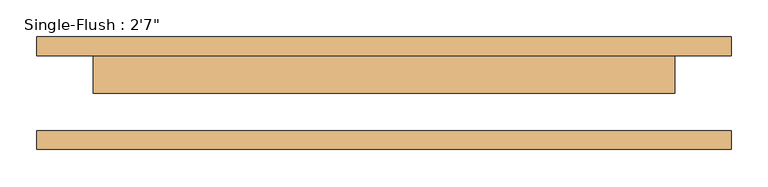
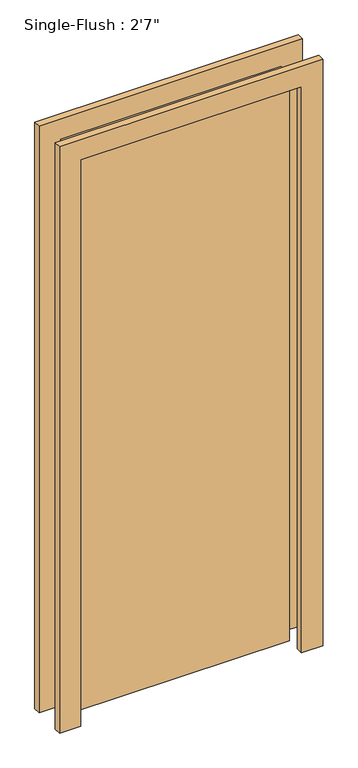
"""IFC4 building model written with IfcOpenShell, lengths in millimetres: door geometry."""

from ifc_helpers import new_model, si_unit, frame, origin, origin_with_axes, place, context, project, spatial, polyline, outline, extrude, source, transform, mapped, element, save


def door_c0900716(model_context):
    return source(origin(), model_context, "Body", "SweptSolid", [
        extrude(outline(polyline([(2209.8, -469.9), (0.0, -469.9), (0.0, -393.7), (2133.6, -393.7), (2133.6, 393.7), (0.0, 393.7), (0.0, 469.9), (2209.8, 469.9), (2209.8, -469.9)])), frame((0.0, 50.8, 0.0), z_axis=(0.0, 1.0, 0.0), x_axis=(0.0, 0.0, 1.0)), (0.0, 0.0, 1.0), 25.4),
        extrude(outline(polyline([(2209.8, 469.9), (2209.8, -469.9), (0.0, -469.9), (0.0, -393.7), (2133.6, -393.7), (2133.6, 393.7), (0.0, 393.7), (0.0, 469.9), (2209.8, 469.9)])), frame((0.0, -76.2, 0.0), z_axis=(0.0, 1.0, 0.0), x_axis=(0.0, 0.0, 1.0)), (0.0, 0.0, 1.0), 25.4),
        extrude(outline(polyline([(393.7, 0.0), (-393.7, 0.0), (-393.7, 50.8), (393.7, 50.8), (393.7, 0.0)])), origin_with_axes(), (0.0, 0.0, 1.0), 2133.6),
    ])


if __name__ == "__main__":
    model = new_model("IFC4")
    model_context = context("Model", 3, world=origin())
    ifc_project = project(units=[si_unit("LENGTHUNIT", "METRE", prefix="MILLI")], contexts=[model_context])
    site = spatial("IfcSite", under=ifc_project)
    building = spatial("IfcBuilding", under=site)
    placement = place(None, origin())
    door_shape = door_c0900716(model_context)
    element("IfcDoor", 1, ObjectType="Single-Flush : 2'7\"", at=placement, inside=building, context=model_context, shape_type="MappedRepresentation", body=[
        mapped(door_shape, transform((0.0, 0.0, 0.0), x_axis=(1.0, 0.0, 0.0), y_axis=(0.0, 1.0, 0.0), z_axis=(0.0, 0.0, 1.0))),
    ])
    save(model, "model.ifc")

# Revit data of these elements
# Type "Single-Flush : 2'7\""
#   Type Mark = "8"
#   Construction Type Id = "MDOOR"
#   Assembly Code = "C1020"
#   Analytic Construction = "Metal"
#   Thickness = 0' - 2"
#   Heat Transfer Coefficient (U) = 0.651978 BTU/(h·ft²·°F)
#   Height = 7' - 0"
#   Trim Projection Ext = 0' - 1"
#   Trim Projection Int = 0' - 1"
#   Trim Width = 0' - 3"
#   Width = 2' - 7"
#   Define Thermal Properties by = 1
#   Door Material = Door - Panel
#   Frame Material = Door - Frame
#   Visual Light Transmittance = 0
#   Solar Heat Gain Coefficient = 0
#   Function = (empty or 0)
#   Wall Closure = (empty or 0)
# Element 1 (IfcDoor, "Single-Flush : 2'7\"")
#   Materials on its faces: "Door - Frame", "Door - Panel"
# Materials
#   "Door - Panel": class "Wood", colour RGB 210 159 95, transparency 0, Cost = 0
#   "Door - Frame": colour RGB 118 70 51, transparency 0, Cost = 0
